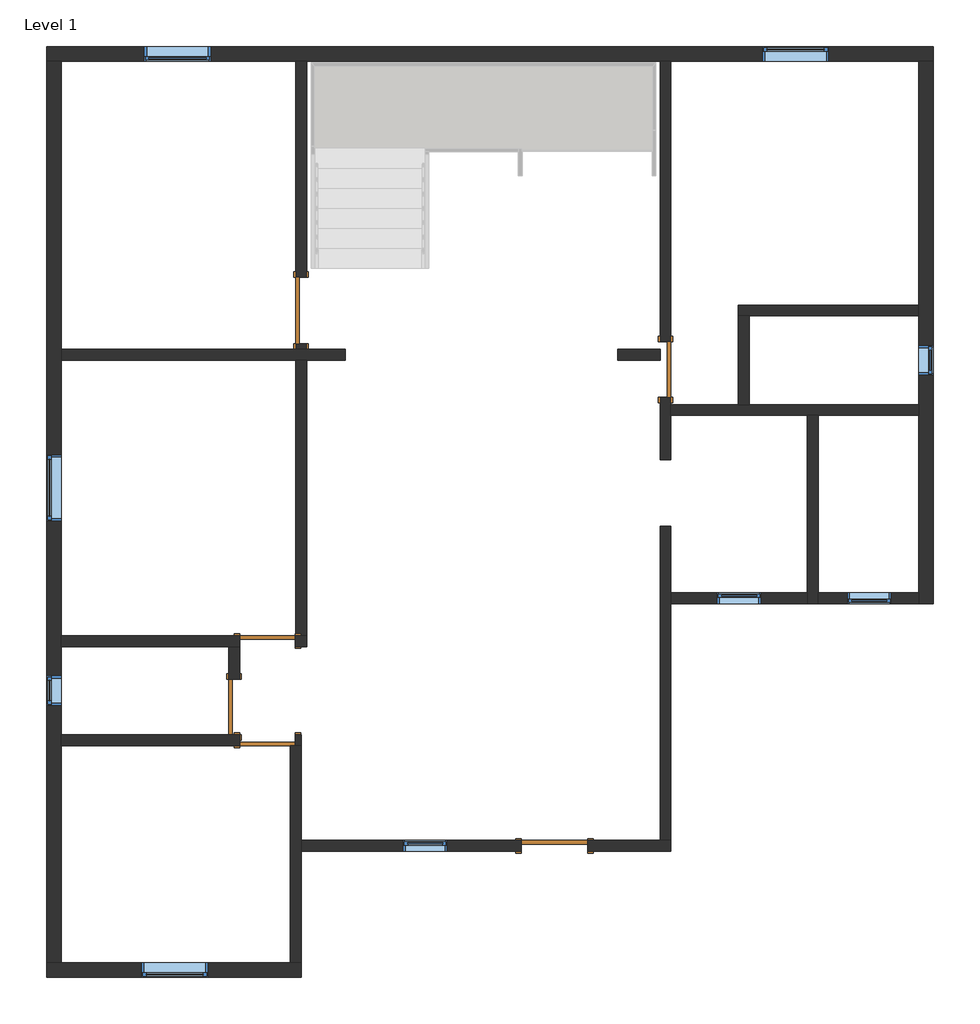
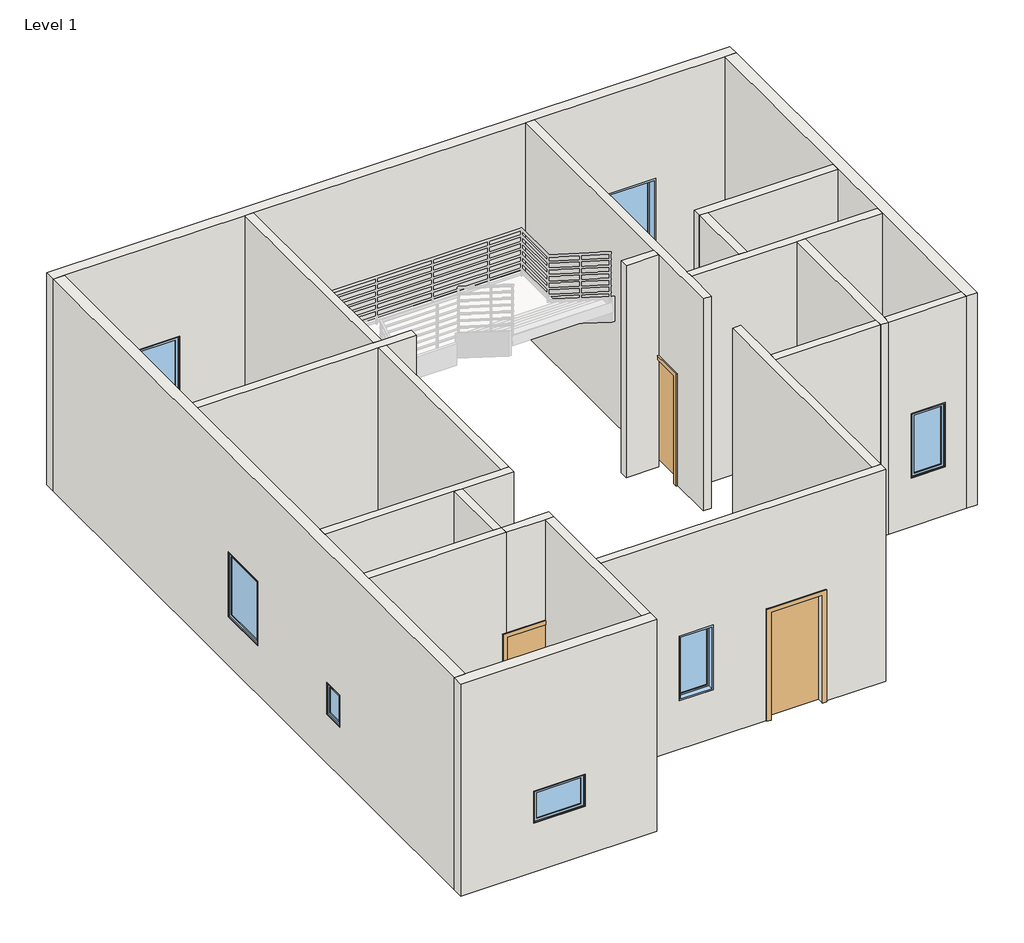
# One storey, part 1 of 3: 22 walls, 9 windows, 6 doors.
"""IFC4 building model written with IfcOpenShell, lengths in millimetres."""

from ifc_helpers import new_model, si_unit, frame, origin, origin_with_axes, place, context, project, spatial, polyline, outline, extrude, faceted_brep, transform, mapped, element, save
from components import m_single_flush_0762_x_2032mm_3f592dcc, m_single_flush_0762_x_2032mm_ffa3ef71, m_single_flush_0915_x_2032mm_d0c19338, m_single_flush_0915_x_2134mm_f3d7f739, m_fixed_0406_x_0610mm_8205b201, m_fixed_0610_x_1220mm_1758882d, m_fixed_0915_x_0610mm_70a843a6, m_fixed_0915_x_1220mm_488fb2fb

model = new_model("IFC4")

# Units and contexts
model_context = context("Model", 3, world=origin())
ifc_project = project(units=[si_unit("LENGTHUNIT", "METRE", prefix="MILLI")], contexts=[model_context])

# Site, building, storey
site = spatial("IfcSite", under=ifc_project)
building = spatial("IfcBuilding", under=site)
storey = spatial("IfcBuildingStorey", under=building, Name="Level 1", Elevation=0.0)

# Doors
placement = place(None, origin())
m_single_flush_0762_x_2032mm_shape = m_single_flush_0762_x_2032mm_3f592dcc(model_context)
element("IfcDoor", 1, ObjectType="M_Single-Flush : 0762 x 2032mm", at=placement, inside=storey, context=model_context, shape_type="MappedRepresentation", body=[
    mapped(m_single_flush_0762_x_2032mm_shape, transform((2439.4843899, 7347.685068, 0.0), x_axis=(0.0, -1.0, 0.0), y_axis=(1.0, 0.0, 0.0), z_axis=(0.0, 0.0, 1.0))),
])
element("IfcDoor", 2, ObjectType="M_Single-Flush : 0762 x 2032mm", at=placement, inside=storey, context=model_context, shape_type="MappedRepresentation", body=[
    mapped(m_single_flush_0762_x_2032mm_shape, transform((-3031.8906101, 3613.885068, 0.0), x_axis=(1.0, 0.0, 0.0), y_axis=(0.0, 1.0, 0.0), z_axis=(0.0, 0.0, 1.0))),
])
m_single_flush_0762_x_2032mm_2_shape = m_single_flush_0762_x_2032mm_ffa3ef71(model_context)
element("IfcDoor", 3, ObjectType="M_Single-Flush : 0762 x 2032mm", at=placement, inside=storey, context=model_context, shape_type="MappedRepresentation", body=[
    mapped(m_single_flush_0762_x_2032mm_2_shape, transform((-3492.2656101, 2707.035068, 0.0), x_axis=(0.0, -1.0, 0.0), y_axis=(1.0, 0.0, 0.0), z_axis=(0.0, 0.0, 1.0))),
])
element("IfcDoor", 4, ObjectType="M_Single-Flush : 0762 x 2032mm", at=placement, inside=storey, context=model_context, shape_type="MappedRepresentation", body=[
    mapped(m_single_flush_0762_x_2032mm_2_shape, transform((-3031.8906101, 2249.835068, 0.0), x_axis=(1.0, 0.0, 0.0), y_axis=(0.0, 1.0, 0.0), z_axis=(0.0, 0.0, 1.0))),
])
m_single_flush_0915_x_2032mm_shape = m_single_flush_0915_x_2032mm_d0c19338(model_context)
element("IfcDoor", 5, ObjectType="M_Single-Flush : 0915 x 2032mm", at=placement, inside=storey, context=model_context, shape_type="MappedRepresentation", body=[
    mapped(m_single_flush_0915_x_2032mm_shape, transform((915.4843899, 797.260068, 0.0), x_axis=(1.0, 0.0, 0.0), y_axis=(0.0, 1.0, 0.0), z_axis=(0.0, 0.0, 1.0))),
])
m_single_flush_0915_x_2134mm_shape = m_single_flush_0915_x_2134mm_f3d7f739(model_context)
element("IfcDoor", 6, ObjectType="M_Single-Flush : 0915 x 2134mm", at=placement, inside=storey, context=model_context, shape_type="MappedRepresentation", body=[
    mapped(m_single_flush_0915_x_2134mm_shape, transform((-2571.5156101, 8160.485068, 0.0), x_axis=(0.0, -1.0, 0.0), y_axis=(1.0, 0.0, 0.0), z_axis=(0.0, 0.0, 1.0))),
])

# Walls
element("IfcWall", 7, ObjectType="Generic - 150mm", at=placement, inside=storey, context=model_context, shape_type="Brep", body=[
    faceted_brep([(-5872.3156101, 7475.885068, 0.0), (-2646.5156101, 7475.885068, 0.0), (-2496.5156101, 7475.885068, 0.0), (-1963.1156101, 7475.885068, 0.0), (-1963.1156101, 7475.885068, 4000.0), (-2496.5156101, 7475.885068, 4000.0), (-2646.5156101, 7475.885068, 4000.0), (-5872.3156101, 7475.885068, 4000.0), (-5872.3156101, 7625.885068, 0.0), (-5872.3156101, 7625.885068, 4000.0), (-2646.5156101, 7625.885068, 4000.0), (-2496.5156101, 7625.885068, 4000.0), (-1963.1156101, 7625.885068, 4000.0), (-1963.1156101, 7625.885068, 0.0), (-2496.5156101, 7625.885068, 0.0), (-2646.5156101, 7625.885068, 0.0)], [[[0, 1, 2, 3, 4, 5, 6, 7]], [[8, 9, 10, 11, 12, 13, 14, 15]], [[3, 2, 1, 0, 8, 15, 14, 13]], [[4, 3, 13, 12]], [[7, 6, 5, 4, 12, 11, 10, 9]], [[0, 7, 9, 8]]]),
])
element("IfcWall", 8, ObjectType="Generic - 150mm", at=placement, inside=storey, context=model_context, shape_type="SweptSolid", body=[
    extrude(outline(polyline([(7702.985068, 2134.0), (7702.985068, 0.0), (7625.885068, 0.0), (7625.885068, 4000.0), (11589.885068, 4000.0), (11589.885068, 0.0), (8617.985068, 0.0), (8617.985068, 2134.0), (7702.985068, 2134.0)])), frame((-2646.5156101, 0.0, 0.0), z_axis=(1.0, 0.0, 0.0), x_axis=(0.0, 1.0, 0.0)), (0.0, 0.0, 1.0), 150.0),
])
element("IfcWall", 9, ObjectType="Generic - 150mm", at=placement, inside=storey, context=model_context, shape_type="Brep", body=[
    faceted_brep([(2364.4843899, 6966.685068, 2032.0), (2364.4843899, 6966.685068, 0.0), (2364.4843899, 6106.685068, 0.0), (2364.4843899, 6106.685068, 4000.0), (2364.4843899, 7475.885068, 4000.0), (2364.4843899, 7625.885068, 4000.0), (2364.4843899, 11589.885068, 4000.0), (2364.4843899, 11589.885068, 0.0), (2364.4843899, 7728.685068, 0.0), (2364.4843899, 7728.685068, 2032.0), (2514.4843899, 6106.685068, 0.0), (2514.4843899, 6716.285068, 0.0), (2514.4843899, 6866.285068, 0.0), (2514.4843899, 6966.685068, 0.0), (2514.4843899, 6966.685068, 2032.0), (2514.4843899, 7728.685068, 2032.0), (2514.4843899, 7728.685068, 0.0), (2514.4843899, 11589.885068, 0.0), (2514.4843899, 11589.885068, 4000.0), (2514.4843899, 6866.285068, 4000.0), (2514.4843899, 6716.285068, 4000.0), (2514.4843899, 6106.685068, 4000.0)], [[[0, 1, 2, 3, 4, 5, 6, 7, 8, 9]], [[10, 11, 12, 13, 14, 15, 16, 17, 18, 19, 20, 21]], [[8, 7, 17, 16]], [[2, 1, 13, 12, 11, 10]], [[3, 2, 10, 21]], [[6, 5, 4, 3, 21, 20, 19, 18]], [[7, 6, 18, 17]], [[14, 13, 1, 0]], [[15, 14, 0, 9]], [[16, 15, 9, 8]]]),
])
element("IfcWall", 10, ObjectType="Generic - 150mm", at=placement, inside=storey, context=model_context, shape_type="Brep", body=[
    faceted_brep([(3439.6343899, 8085.485068, 0.0), (3589.6343899, 8085.485068, 0.0), (5919.6843899, 8085.485068, 0.0), (5919.6843899, 8085.485068, 4000.0), (3589.6343899, 8085.485068, 4000.0), (3439.6343899, 8085.485068, 4000.0), (3439.6343899, 8235.485068, 0.0), (3439.6343899, 8235.485068, 4000.0), (5919.6843899, 8235.485068, 4000.0), (5919.6843899, 8235.485068, 0.0)], [[[0, 1, 2, 3, 4, 5]], [[6, 7, 8, 9]], [[2, 1, 0, 6, 9]], [[5, 4, 3, 8, 7]], [[3, 2, 9, 8]], [[0, 5, 7, 6]]]),
])
element("IfcWall", 11, ObjectType="Generic - 150mm", at=placement, inside=storey, context=model_context, shape_type="Brep", body=[
    faceted_brep([(-2496.5156101, 3688.885068, 0.0), (-2646.5156101, 3688.885068, 0.0), (-2650.8906101, 3688.885068, 0.0), (-2650.8906101, 3688.885068, 2032.0), (-3412.8906101, 3688.885068, 2032.0), (-3412.8906101, 3688.885068, 0.0), (-5872.3156101, 3688.885068, 0.0), (-5872.3156101, 3688.885068, 4000.0), (-2646.5156101, 3688.885068, 4000.0), (-2496.5156101, 3688.885068, 4000.0), (-2650.8906101, 3538.885068, 2032.0), (-2650.8906101, 3538.885068, 0.0), (-2496.5156101, 3538.885068, 0.0), (-2496.5156101, 3538.885068, 4000.0), (-3417.2656101, 3538.885068, 4000.0), (-3567.2656101, 3538.885068, 4000.0), (-5872.3156101, 3538.885068, 4000.0), (-5872.3156101, 3538.885068, 0.0), (-3567.2656101, 3538.885068, 0.0), (-3417.2656101, 3538.885068, 0.0), (-3412.8906101, 3538.885068, 0.0), (-3412.8906101, 3538.885068, 2032.0)], [[[0, 1, 2, 3, 4, 5, 6, 7, 8, 9]], [[10, 11, 12, 13, 14, 15, 16, 17, 18, 19, 20, 21]], [[12, 11, 2, 1, 0]], [[20, 19, 18, 17, 6, 5]], [[9, 8, 7, 16, 15, 14, 13]], [[7, 6, 17, 16]], [[0, 9, 13, 12]], [[3, 2, 11, 10]], [[4, 3, 10, 21]], [[5, 4, 21, 20]]]),
])
element("IfcWall", 12, ObjectType="Generic - 150mm", at=placement, inside=storey, context=model_context, shape_type="SweptSolid", body=[
    extrude(outline(polyline([(3439.6343899, 6866.285068), (3439.6343899, 8085.485068), (3589.6343899, 8085.485068), (3589.6343899, 6866.285068), (3439.6343899, 6866.285068)])), origin_with_axes(), (0.0, 0.0, 1.0), 4000.0),
])
element("IfcWall", 13, ObjectType="Generic - 150mm", at=placement, inside=storey, context=model_context, shape_type="Brep", body=[
    faceted_brep([(2514.4843899, 6716.285068, 0.0), (4390.1343899, 6716.285068, 0.0), (4540.1343899, 6716.285068, 0.0), (5919.6843899, 6716.285068, 0.0), (5919.6843899, 6716.285068, 4000.0), (4540.1343899, 6716.285068, 4000.0), (4390.1343899, 6716.285068, 4000.0), (2514.4843899, 6716.285068, 4000.0), (2514.4843899, 6866.285068, 0.0), (2514.4843899, 6866.285068, 4000.0), (3439.6343899, 6866.285068, 4000.0), (3589.6343899, 6866.285068, 4000.0), (5919.6843899, 6866.285068, 4000.0), (5919.6843899, 6866.285068, 0.0), (3589.6343899, 6866.285068, 0.0), (3439.6343899, 6866.285068, 0.0)], [[[0, 1, 2, 3, 4, 5, 6, 7]], [[8, 9, 10, 11, 12, 13, 14, 15]], [[3, 2, 1, 0, 8, 15, 14, 13]], [[7, 6, 5, 4, 12, 11, 10, 9]], [[4, 3, 13, 12]], [[0, 7, 9, 8]]]),
])
element("IfcWall", 14, ObjectType="Generic - 150mm", at=placement, inside=storey, context=model_context, shape_type="Brep", body=[
    faceted_brep([(4390.1343899, 6716.285068, 0.0), (4390.1343899, 4277.885068, 0.0), (4390.1343899, 4127.885068, 0.0), (4390.1343899, 4127.885068, 4000.0), (4390.1343899, 4277.885068, 4000.0), (4390.1343899, 6716.285068, 4000.0), (4540.1343899, 6716.285068, 0.0), (4540.1343899, 6716.285068, 4000.0), (4540.1343899, 4277.885068, 4000.0), (4540.1343899, 4127.885068, 4000.0), (4540.1343899, 4127.885068, 0.0), (4540.1343899, 4277.885068, 0.0)], [[[0, 1, 2, 3, 4, 5]], [[6, 7, 8, 9, 10, 11]], [[2, 1, 0, 6, 11, 10]], [[5, 4, 3, 9, 8, 7]], [[0, 5, 7, 6]], [[3, 2, 10, 9]]]),
])
element("IfcWall", 15, ObjectType="Generic - 150mm", at=placement, inside=storey, context=model_context, shape_type="SweptSolid", body=[
    extrude(outline(polyline([(0.0, 4540.1343899), (0.0, 5919.6843899), (4000.0, 5919.6843899), (4000.0, 4540.1343899), (0.0, 4540.1343899)]), holes=[polyline([(915.0, 5547.4093899), (915.0, 4937.4093899), (2135.0, 4937.4093899), (2135.0, 5547.4093899), (915.0, 5547.4093899)])]), frame((0.0, 4127.885068, 0.0), z_axis=(0.0, 1.0, 0.0), x_axis=(0.0, 0.0, 1.0)), (0.0, 0.0, 1.0), 150.0),
])
element("IfcWall", 16, ObjectType="Generic - 150mm", at=placement, inside=storey, context=model_context, shape_type="SweptSolid", body=[
    extrude(outline(polyline([(0.0, 4390.1343899), (4000.0, 4390.1343899), (4000.0, 2514.4843899), (0.0, 2514.4843899), (0.0, 4390.1343899)]), holes=[polyline([(915.0, 3147.3093899), (2135.0, 3147.3093899), (2135.0, 3757.3093899), (915.0, 3757.3093899), (915.0, 3147.3093899)])]), frame((0.0, 4127.885068, 0.0), z_axis=(0.0, 1.0, 0.0), x_axis=(0.0, 0.0, 1.0)), (0.0, 0.0, 1.0), 150.0),
])
element("IfcWall", 17, ObjectType="Generic - 150mm", at=placement, inside=storey, context=model_context, shape_type="Brep", body=[
    faceted_brep([(2514.4843899, 872.260068, 0.0), (2514.4843899, 4127.885068, 0.0), (2514.4843899, 4277.885068, 0.0), (2514.4843899, 5194.685068, 0.0), (2514.4843899, 5194.685068, 4000.0), (2514.4843899, 4277.885068, 4000.0), (2514.4843899, 4127.885068, 4000.0), (2514.4843899, 872.260068, 4000.0), (2364.4843899, 872.260068, 0.0), (2364.4843899, 872.260068, 4000.0), (2364.4843899, 5194.685068, 4000.0), (2364.4843899, 5194.685068, 0.0)], [[[0, 1, 2, 3, 4, 5, 6, 7]], [[8, 9, 10, 11]], [[3, 2, 1, 0, 8, 11]], [[4, 3, 11, 10]], [[7, 6, 5, 4, 10, 9]], [[0, 7, 9, 8]]]),
])
element("IfcWall", 18, ObjectType="Generic - 150mm", at=placement, inside=storey, context=model_context, shape_type="Brep", body=[
    faceted_brep([(-5872.3156101, 2174.835068, 0.0), (-3417.2656101, 2174.835068, 0.0), (-3417.2656101, 2174.835068, 4000.0), (-5872.3156101, 2174.835068, 4000.0), (-5872.3156101, 2324.835068, 0.0), (-5872.3156101, 2324.835068, 4000.0), (-3567.2656101, 2324.835068, 4000.0), (-3417.2656101, 2324.835068, 4000.0), (-3417.2656101, 2324.835068, 0.0), (-3567.2656101, 2324.835068, 0.0)], [[[0, 1, 2, 3]], [[4, 5, 6, 7, 8, 9]], [[1, 0, 4, 9, 8]], [[3, 2, 7, 6, 5]], [[0, 3, 5, 4]], [[2, 1, 8, 7]]]),
])
element("IfcWall", 19, ObjectType="Generic - 150mm", at=placement, inside=storey, context=model_context, shape_type="SweptSolid", body=[
    extrude(outline(polyline([(2326.035068, 2032.0), (2326.035068, 0.0), (2324.835068, 0.0), (2324.835068, 4000.0), (3538.885068, 4000.0), (3538.885068, 0.0), (3088.035068, 0.0), (3088.035068, 2032.0), (2326.035068, 2032.0)])), frame((-3567.2656101, 0.0, 0.0), z_axis=(1.0, 0.0, 0.0), x_axis=(0.0, 1.0, 0.0)), (0.0, 0.0, 1.0), 150.0),
])
element("IfcWall", 20, ObjectType="Generic - 150mm", at=placement, inside=storey, context=model_context, shape_type="Brep", body=[
    faceted_brep([(-2571.5156101, 2324.835068, 0.0), (-2650.8906101, 2324.835068, 0.0), (-2650.8906101, 2324.835068, 2032.0), (-3412.8906101, 2324.835068, 2032.0), (-3412.8906101, 2324.835068, 0.0), (-3417.2656101, 2324.835068, 0.0), (-3417.2656101, 2324.835068, 4000.0), (-2571.5156101, 2324.835068, 4000.0), (-2650.8906101, 2174.835068, 2032.0), (-2650.8906101, 2174.835068, 0.0), (-2571.5156101, 2174.835068, 0.0), (-2571.5156101, 2174.835068, 4000.0), (-2721.5156101, 2174.835068, 4000.0), (-3417.2656101, 2174.835068, 4000.0), (-3417.2656101, 2174.835068, 0.0), (-3412.8906101, 2174.835068, 0.0), (-3412.8906101, 2174.835068, 2032.0)], [[[0, 1, 2, 3, 4, 5, 6, 7]], [[8, 9, 10, 11, 12, 13, 14, 15, 16]], [[15, 14, 5, 4]], [[10, 9, 1, 0]], [[7, 6, 13, 12, 11]], [[6, 5, 14, 13]], [[0, 7, 11, 10]], [[2, 1, 9, 8]], [[3, 2, 8, 16]], [[4, 3, 16, 15]]]),
])
element("IfcWall", 21, ObjectType="Generic - 150mm", at=placement, inside=storey, context=model_context, shape_type="SweptSolid", body=[
    extrude(outline(polyline([(-2646.5156101, 3688.885068), (-2646.5156101, 7475.885068), (-2496.5156101, 7475.885068), (-2496.5156101, 3688.885068), (-2646.5156101, 3688.885068)])), origin_with_axes(), (0.0, 0.0, 1.0), 4000.0),
])
element("IfcWall", 22, ObjectType="Generic - 150mm", at=placement, inside=storey, context=model_context, shape_type="Brep", body=[
    faceted_brep([(-2721.5156101, 2174.835068, 0.0), (-2721.5156101, -811.714932, 0.0), (-2721.5156101, -811.714932, 4000.0), (-2721.5156101, 2174.835068, 4000.0), (-2571.5156101, 2174.835068, 0.0), (-2571.5156101, 2174.835068, 4000.0), (-2571.5156101, 872.260068, 4000.0), (-2571.5156101, 722.260068, 4000.0), (-2571.5156101, -811.714932, 4000.0), (-2571.5156101, -811.714932, 0.0), (-2571.5156101, 722.260068, 0.0), (-2571.5156101, 872.260068, 0.0)], [[[0, 1, 2, 3]], [[4, 5, 6, 7, 8, 9, 10, 11]], [[1, 0, 4, 11, 10, 9]], [[3, 2, 8, 7, 6, 5]], [[0, 3, 5, 4]], [[2, 1, 9, 8]]]),
])
element("IfcWall", 23, ObjectType="Generic - 150mm", at=placement, inside=storey, context=model_context, shape_type="Brep", body=[
    faceted_brep([(1372.9843899, 722.260068, 2032.0), (1372.9843899, 722.260068, 0.0), (2514.4843899, 722.260068, 0.0), (2514.4843899, 722.260068, 4000.0), (-2571.5156101, 722.260068, 4000.0), (-2571.5156101, 722.260068, 0.0), (457.9843899, 722.260068, 0.0), (457.9843899, 722.260068, 2032.0), (-1170.5156101, 722.260068, 915.0), (-1170.5156101, 722.260068, 2135.0), (-560.5156101, 722.260068, 2135.0), (-560.5156101, 722.260068, 915.0), (2514.4843899, 872.260068, 0.0), (2364.4843899, 872.260068, 0.0), (1372.9843899, 872.260068, 0.0), (1372.9843899, 872.260068, 2032.0), (457.9843899, 872.260068, 2032.0), (457.9843899, 872.260068, 0.0), (-2571.5156101, 872.260068, 0.0), (-2571.5156101, 872.260068, 4000.0), (2364.4843899, 872.260068, 4000.0), (2514.4843899, 872.260068, 4000.0), (-1170.5156101, 872.260068, 915.0), (-560.5156101, 872.260068, 915.0), (-560.5156101, 872.260068, 2135.0), (-1170.5156101, 872.260068, 2135.0)], [[[0, 1, 2, 3, 4, 5, 6, 7], [8, 9, 10, 11]], [[12, 13, 14, 15, 16, 17, 18, 19, 20, 21], [22, 23, 24, 25]], [[6, 5, 18, 17]], [[2, 1, 14, 13, 12]], [[4, 3, 21, 20, 19]], [[5, 4, 19, 18]], [[3, 2, 12, 21]], [[15, 14, 1, 0]], [[16, 15, 0, 7]], [[17, 16, 7, 6]], [[9, 8, 22, 25]], [[10, 9, 25, 24]], [[11, 10, 24, 23]], [[8, 11, 23, 22]]]),
])
element("IfcWall", 24, ObjectType="Generic - 150mm", at=placement, inside=storey, context=model_context, shape_type="SweptSolid", body=[
    extrude(outline(polyline([(1780.2843899, 7625.885068), (2364.4843899, 7625.885068), (2364.4843899, 7475.885068), (1780.2843899, 7475.885068), (1780.2843899, 7625.885068)])), origin_with_axes(), (0.0, 0.0, 1.0), 4000.0),
])
element("IfcWall", 25, ObjectType="Generic - 200mm", at=placement, inside=storey, context=model_context, shape_type="Brep", body=[
    faceted_brep([(-6072.3156101, 11589.885068, 0.0), (-5872.3156101, 11589.885068, 0.0), (-2646.5156101, 11589.885068, 0.0), (-2496.5156101, 11589.885068, 0.0), (2364.4843899, 11589.885068, 0.0), (2514.4843899, 11589.885068, 0.0), (5919.6843899, 11589.885068, 0.0), (6119.6843899, 11589.885068, 0.0), (6119.6843899, 11589.885068, 4000.0), (5919.6843899, 11589.885068, 4000.0), (2514.4843899, 11589.885068, 4000.0), (2364.4843899, 11589.885068, 4000.0), (-2496.5156101, 11589.885068, 4000.0), (-2646.5156101, 11589.885068, 4000.0), (-5872.3156101, 11589.885068, 4000.0), (-6072.3156101, 11589.885068, 4000.0), (-3814.4156101, 11589.885068, 915.0), (-4729.4156101, 11589.885068, 915.0), (-4729.4156101, 11589.885068, 2135.0), (-3814.4156101, 11589.885068, 2135.0), (3772.0843899, 11589.885068, 915.0), (3772.0843899, 11589.885068, 2135.0), (4687.0843899, 11589.885068, 2135.0), (4687.0843899, 11589.885068, 915.0), (-6072.3156101, 11789.885068, 0.0), (-6072.3156101, 11789.885068, 4000.0), (6119.6843899, 11789.885068, 4000.0), (6119.6843899, 11789.885068, 0.0), (-3814.4156101, 11789.885068, 915.0), (-3814.4156101, 11789.885068, 2135.0), (-4729.4156101, 11789.885068, 2135.0), (-4729.4156101, 11789.885068, 915.0), (3772.0843899, 11789.885068, 915.0), (4687.0843899, 11789.885068, 915.0), (4687.0843899, 11789.885068, 2135.0), (3772.0843899, 11789.885068, 2135.0)], [[[0, 1, 2, 3, 4, 5, 6, 7, 8, 9, 10, 11, 12, 13, 14, 15], [16, 17, 18, 19], [20, 21, 22, 23]], [[24, 25, 26, 27], [28, 29, 30, 31], [32, 33, 34, 35]], [[7, 6, 5, 4, 3, 2, 1, 0, 24, 27]], [[15, 14, 13, 12, 11, 10, 9, 8, 26, 25]], [[8, 7, 27, 26]], [[0, 15, 25, 24]], [[29, 28, 16, 19]], [[30, 29, 19, 18]], [[31, 30, 18, 17]], [[28, 31, 17, 16]], [[21, 20, 32, 35]], [[22, 21, 35, 34]], [[23, 22, 34, 33]], [[20, 23, 33, 32]]]),
])
element("IfcWall", 26, ObjectType="Generic - 200mm", at=placement, inside=storey, context=model_context, shape_type="Brep", body=[
    faceted_brep([(5919.6843899, 11589.885068, 0.0), (5919.6843899, 8235.485068, 0.0), (5919.6843899, 8085.485068, 0.0), (5919.6843899, 6866.285068, 0.0), (5919.6843899, 6716.285068, 0.0), (5919.6843899, 4277.885068, 0.0), (5919.6843899, 4127.885068, 0.0), (5919.6843899, 4127.885068, 4000.0), (5919.6843899, 4277.885068, 4000.0), (5919.6843899, 6716.285068, 4000.0), (5919.6843899, 6866.285068, 4000.0), (5919.6843899, 8085.485068, 4000.0), (5919.6843899, 8235.485068, 4000.0), (5919.6843899, 11589.885068, 4000.0), (5919.6843899, 7678.885068, 915.0), (5919.6843899, 7678.885068, 1525.0), (5919.6843899, 7272.885068, 1525.0), (5919.6843899, 7272.885068, 915.0), (6119.6843899, 11589.885068, 0.0), (6119.6843899, 11589.885068, 4000.0), (6119.6843899, 4127.885068, 4000.0), (6119.6843899, 4127.885068, 0.0), (6119.6843899, 7678.885068, 915.0), (6119.6843899, 7272.885068, 915.0), (6119.6843899, 7272.885068, 1525.0), (6119.6843899, 7678.885068, 1525.0)], [[[0, 1, 2, 3, 4, 5, 6, 7, 8, 9, 10, 11, 12, 13], [14, 15, 16, 17]], [[18, 19, 20, 21], [22, 23, 24, 25]], [[6, 5, 4, 3, 2, 1, 0, 18, 21]], [[13, 12, 11, 10, 9, 8, 7, 20, 19]], [[0, 13, 19, 18]], [[7, 6, 21, 20]], [[15, 14, 22, 25]], [[16, 15, 25, 24]], [[17, 16, 24, 23]], [[14, 17, 23, 22]]]),
])
element("IfcWall", 27, ObjectType="Generic - 200mm", at=placement, inside=storey, context=model_context, shape_type="Brep", body=[
    faceted_brep([(-2571.5156101, -811.714932, 0.0), (-2721.5156101, -811.714932, 0.0), (-5872.3156101, -811.714932, 0.0), (-6072.3156101, -811.714932, 0.0), (-6072.3156101, -811.714932, 4000.0), (-5872.3156101, -811.714932, 4000.0), (-2721.5156101, -811.714932, 4000.0), (-2571.5156101, -811.714932, 4000.0), (-3851.9156101, -811.714932, 915.0), (-3851.9156101, -811.714932, 1525.0), (-4766.9156101, -811.714932, 1525.0), (-4766.9156101, -811.714932, 915.0), (-2571.5156101, -1011.714932, 0.0), (-2571.5156101, -1011.714932, 4000.0), (-6072.3156101, -1011.714932, 4000.0), (-6072.3156101, -1011.714932, 0.0), (-3851.9156101, -1011.714932, 915.0), (-4766.9156101, -1011.714932, 915.0), (-4766.9156101, -1011.714932, 1525.0), (-3851.9156101, -1011.714932, 1525.0)], [[[0, 1, 2, 3, 4, 5, 6, 7], [8, 9, 10, 11]], [[12, 13, 14, 15], [16, 17, 18, 19]], [[3, 2, 1, 0, 12, 15]], [[7, 6, 5, 4, 14, 13]], [[4, 3, 15, 14]], [[0, 7, 13, 12]], [[9, 8, 16, 19]], [[10, 9, 19, 18]], [[11, 10, 18, 17]], [[8, 11, 17, 16]]]),
])
element("IfcWall", 28, ObjectType="Generic - 200mm", at=placement, inside=storey, context=model_context, shape_type="Brep", body=[
    faceted_brep([(-5872.3156101, -811.714932, 0.0), (-5872.3156101, 2174.835068, 0.0), (-5872.3156101, 2324.835068, 0.0), (-5872.3156101, 3538.885068, 0.0), (-5872.3156101, 3688.885068, 0.0), (-5872.3156101, 7475.885068, 0.0), (-5872.3156101, 7625.885068, 0.0), (-5872.3156101, 11589.885068, 0.0), (-5872.3156101, 11589.885068, 4000.0), (-5872.3156101, 7625.885068, 4000.0), (-5872.3156101, 7475.885068, 4000.0), (-5872.3156101, 3688.885068, 4000.0), (-5872.3156101, 3538.885068, 4000.0), (-5872.3156101, 2324.835068, 4000.0), (-5872.3156101, 2174.835068, 4000.0), (-5872.3156101, -811.714932, 4000.0), (-5872.3156101, 2728.860068, 915.0), (-5872.3156101, 2728.860068, 1525.0), (-5872.3156101, 3134.860068, 1525.0), (-5872.3156101, 3134.860068, 915.0), (-5872.3156101, 5264.585068, 915.0), (-5872.3156101, 5264.585068, 2135.0), (-5872.3156101, 6179.585068, 2135.0), (-5872.3156101, 6179.585068, 915.0), (-6072.3156101, -811.714932, 0.0), (-6072.3156101, -811.714932, 4000.0), (-6072.3156101, 11589.885068, 4000.0), (-6072.3156101, 11589.885068, 0.0), (-6072.3156101, 2728.860068, 915.0), (-6072.3156101, 3134.860068, 915.0), (-6072.3156101, 3134.860068, 1525.0), (-6072.3156101, 2728.860068, 1525.0), (-6072.3156101, 5264.585068, 915.0), (-6072.3156101, 6179.585068, 915.0), (-6072.3156101, 6179.585068, 2135.0), (-6072.3156101, 5264.585068, 2135.0)], [[[0, 1, 2, 3, 4, 5, 6, 7, 8, 9, 10, 11, 12, 13, 14, 15], [16, 17, 18, 19], [20, 21, 22, 23]], [[24, 25, 26, 27], [28, 29, 30, 31], [32, 33, 34, 35]], [[7, 6, 5, 4, 3, 2, 1, 0, 24, 27]], [[15, 14, 13, 12, 11, 10, 9, 8, 26, 25]], [[0, 15, 25, 24]], [[8, 7, 27, 26]], [[17, 16, 28, 31]], [[18, 17, 31, 30]], [[19, 18, 30, 29]], [[16, 19, 29, 28]], [[21, 20, 32, 35]], [[22, 21, 35, 34]], [[23, 22, 34, 33]], [[20, 23, 33, 32]]]),
])

# Windows
m_fixed_0406_x_0610mm_shape = m_fixed_0406_x_0610mm_8205b201(model_context)
element("IfcWindow", 29, ObjectType="M_Fixed : 0406 x 0610mm", at=placement, inside=storey, context=model_context, shape_type="MappedRepresentation", body=[
    mapped(m_fixed_0406_x_0610mm_shape, transform((-5959.3156101, 2931.860068, 0.0), x_axis=(0.0, 1.0, 0.0), y_axis=(-1.0, 0.0, 0.0), z_axis=(0.0, 0.0, 1.0))),
])
element("IfcWindow", 30, ObjectType="M_Fixed : 0406 x 0610mm", at=placement, inside=storey, context=model_context, shape_type="MappedRepresentation", body=[
    mapped(m_fixed_0406_x_0610mm_shape, transform((6006.6843899, 7475.885068, 0.0), x_axis=(0.0, -1.0, 0.0), y_axis=(1.0, 0.0, 0.0), z_axis=(0.0, 0.0, 1.0))),
])
m_fixed_0610_x_1220mm_shape = m_fixed_0610_x_1220mm_1758882d(model_context)
element("IfcWindow", 31, ObjectType="M_Fixed : 0610 x 1220mm", at=placement, inside=storey, context=model_context, shape_type="MappedRepresentation", body=[
    mapped(m_fixed_0610_x_1220mm_shape, transform((3452.3093899, 4189.885068, 0.0), x_axis=(1.0, 0.0, 0.0), y_axis=(0.0, 1.0, 0.0), z_axis=(0.0, 0.0, 1.0))),
])
element("IfcWindow", 32, ObjectType="M_Fixed : 0610 x 1220mm", at=placement, inside=storey, context=model_context, shape_type="MappedRepresentation", body=[
    mapped(m_fixed_0610_x_1220mm_shape, transform((5242.4093899, 4215.885068, 0.0), x_axis=(-1.0, 0.0, 0.0), y_axis=(0.0, -1.0, 0.0), z_axis=(0.0, 0.0, 1.0))),
])
element("IfcWindow", 33, ObjectType="M_Fixed : 0610 x 1220mm", at=placement, inside=storey, context=model_context, shape_type="MappedRepresentation", body=[
    mapped(m_fixed_0610_x_1220mm_shape, transform((-865.5156101, 784.260068, 0.0), x_axis=(1.0, 0.0, 0.0), y_axis=(0.0, 1.0, 0.0), z_axis=(0.0, 0.0, 1.0))),
])
m_fixed_0915_x_0610mm_shape = m_fixed_0915_x_0610mm_70a843a6(model_context)
element("IfcWindow", 34, ObjectType="M_Fixed : 0915 x 0610mm", at=placement, inside=storey, context=model_context, shape_type="MappedRepresentation", body=[
    mapped(m_fixed_0915_x_0610mm_shape, transform((-4309.4156101, -898.714932, 0.0), x_axis=(-1.0, 0.0, 0.0), y_axis=(0.0, -1.0, 0.0), z_axis=(0.0, 0.0, 1.0))),
])
m_fixed_0915_x_1220mm_shape = m_fixed_0915_x_1220mm_488fb2fb(model_context)
element("IfcWindow", 35, ObjectType="M_Fixed : 0915 x 1220mm", at=placement, inside=storey, context=model_context, shape_type="MappedRepresentation", body=[
    mapped(m_fixed_0915_x_1220mm_shape, transform((-5959.3156101, 5722.085068, 0.0), x_axis=(0.0, 1.0, 0.0), y_axis=(-1.0, 0.0, 0.0), z_axis=(0.0, 0.0, 1.0))),
])
element("IfcWindow", 36, ObjectType="M_Fixed : 0915 x 1220mm", at=placement, inside=storey, context=model_context, shape_type="MappedRepresentation", body=[
    mapped(m_fixed_0915_x_1220mm_shape, transform((-4271.9156101, 11702.885068, 0.0), x_axis=(-1.0, 0.0, 0.0), y_axis=(0.0, -1.0, 0.0), z_axis=(0.0, 0.0, 1.0))),
])
element("IfcWindow", 37, ObjectType="M_Fixed : 0915 x 1220mm", at=placement, inside=storey, context=model_context, shape_type="MappedRepresentation", body=[
    mapped(m_fixed_0915_x_1220mm_shape, transform((4229.5843899, 11676.885068, 0.0), x_axis=(1.0, 0.0, 0.0), y_axis=(0.0, 1.0, 0.0), z_axis=(0.0, 0.0, 1.0))),
])

save(model, "model.ifc")

# Revit data of these elements
# Type "M_Single-Flush : 0762 x 2032mm"
#   Type Mark = "19"
#   Thickness = 51 mm
#   Height = 2032 mm
#   Trim Projection Ext = 25 mm
#   Trim Projection Int = 25 mm
#   Trim Width = 76 mm
#   Width = 762 mm
#   Door Material = Door - Panel
#   Frame Material = Door - Frame
#   Function = (empty or 0)
#   Wall Closure = (empty or 0)
# Type "M_Single-Flush : 0915 x 2032mm"
#   Type Mark = "20"
#   Thickness = 51 mm
#   Height = 2032 mm
#   Trim Projection Ext = 25 mm
#   Trim Projection Int = 25 mm
#   Trim Width = 76 mm
#   Width = 915 mm
#   Door Material = Door - Panel
#   Frame Material = Door - Frame
#   Function = (empty or 0)
#   Wall Closure = (empty or 0)
# Type "M_Single-Flush : 0915 x 2134mm"
#   Type Mark = "15"
#   Thickness = 51 mm
#   Height = 2134 mm
#   Trim Projection Ext = 25 mm
#   Trim Projection Int = 25 mm
#   Trim Width = 76 mm
#   Width = 915 mm
#   Door Material = Door - Panel
#   Frame Material = Door - Frame
#   Function = (empty or 0)
#   Wall Closure = (empty or 0)
# Type "Generic - 150mm"
#   Layers, outside or top first: 150 mm no material (function 1)
# Type "Generic - 200mm"
#   Layers, outside or top first: 200 mm no material (function 1)
# Type "M_Fixed : 0406 x 0610mm"
#   Type Mark = "10"
#   Height = 610 mm
#   Default Sill Height = 915 mm
#   Width = 406 mm
#   Window Inset = 19 mm
#   Frame Exterior Material = Sash
#   Frame Interior Material = Sash
#   Glass Pane Material = Glass
#   Sash = Sash
#   Wall Closure = (empty or 0)
# Type "M_Fixed : 0610 x 1220mm"
#   Type Mark = "13"
#   Height = 1220 mm
#   Default Sill Height = 915 mm
#   Width = 610 mm
#   Window Inset = 19 mm
#   Frame Exterior Material = Sash
#   Frame Interior Material = Sash
#   Glass Pane Material = Glass
#   Sash = Sash
#   Wall Closure = (empty or 0)
# Type "M_Fixed : 0915 x 0610mm"
#   Type Mark = "14"
#   Height = 610 mm
#   Default Sill Height = 915 mm
#   Width = 915 mm
#   Window Inset = 19 mm
#   Frame Exterior Material = Sash
#   Frame Interior Material = Sash
#   Glass Pane Material = Glass
#   Sash = Sash
#   Wall Closure = (empty or 0)
# Type "M_Fixed : 0915 x 1220mm"
#   Type Mark = "15"
#   Height = 1220 mm
#   Default Sill Height = 915 mm
#   Width = 915 mm
#   Window Inset = 19 mm
#   Frame Exterior Material = Sash
#   Frame Interior Material = Sash
#   Glass Pane Material = Glass
#   Sash = Sash
#   Wall Closure = (empty or 0)
# Elements 1, 2, 3, 4 (IfcDoor, "M_Single-Flush : 0762 x 2032mm")
#   Phase Created = New Construction
#   Materials on its faces: "Door - Frame", "Door - Panel"
# Element 5 (IfcDoor, "M_Single-Flush : 0915 x 2032mm")
#   Phase Created = New Construction
#   Materials on its faces: "Door - Frame", "Door - Panel"
# Element 6 (IfcDoor, "M_Single-Flush : 0915 x 2134mm")
#   Phase Created = New Construction
#   Materials on its faces: "Door - Frame", "Door - Panel"
# Elements 7, 8, 9, 10, 11, 12, 13, 14, 15, 16, 17, 18, 19, 20, 21, 22, 23, 24 (IfcWall, "Generic - 150mm")
#   Top Offset = 0 mm
#   Base Offset = 0 mm
#   wall height = 4000 mm
#   Phase Created = New Construction
#   Base Constraint = Level 1
#   Top Constraint = Level 2
#   Materials on its faces: "Default Wall"
# Elements 25, 26, 27, 28 (IfcWall, "Generic - 200mm")
#   Top Offset = 0 mm
#   Base Offset = 0 mm
#   wall height = 4000 mm
#   Phase Created = New Construction
#   Base Constraint = Level 1
#   Top Constraint = Level 2
#   Materials on its faces: "Default Wall"
# Element 29 (IfcWindow, "M_Fixed : 0406 x 0610mm")
#   Mark = "6"
#   Phase Created = New Construction
#   Materials on its faces: "Sash", "Glass"
# Element 30 (IfcWindow, "M_Fixed : 0406 x 0610mm")
#   Mark = "7"
#   Phase Created = New Construction
#   Materials on its faces: "Sash", "Glass"
# Element 31 (IfcWindow, "M_Fixed : 0610 x 1220mm")
#   Mark = "11"
#   Phase Created = New Construction
#   Materials on its faces: "Sash", "Glass"
# Element 32 (IfcWindow, "M_Fixed : 0610 x 1220mm")
#   Mark = "12"
#   Phase Created = New Construction
#   Materials on its faces: "Sash", "Glass"
# Element 33 (IfcWindow, "M_Fixed : 0610 x 1220mm")
#   Mark = "13"
#   Phase Created = New Construction
#   Materials on its faces: "Sash", "Glass"
# Element 34 (IfcWindow, "M_Fixed : 0915 x 0610mm")
#   Mark = "14"
#   Phase Created = New Construction
#   Materials on its faces: "Sash", "Glass"
# Element 35 (IfcWindow, "M_Fixed : 0915 x 1220mm")
#   Mark = "8"
#   Phase Created = New Construction
#   Materials on its faces: "Sash", "Glass"
# Element 36 (IfcWindow, "M_Fixed : 0915 x 1220mm")
#   Mark = "9"
#   Phase Created = New Construction
#   Materials on its faces: "Sash", "Glass"
# Element 37 (IfcWindow, "M_Fixed : 0915 x 1220mm")
#   Mark = "10"
#   Phase Created = New Construction
#   Materials on its faces: "Sash", "Glass"
# Materials
#   "Door - Panel": class "Wood", colour RGB 114 82 51, transparency 0
#   "Door - Frame": colour RGB 153 76 43, transparency 0
#   "Sash": class "Wood", colour RGB 136 99 55, transparency 0
#   "Glass": class "Glass", colour RGB 218 227 224, transparency 0.85, Description = "Soda Lime Glass", Cost = 0
#   "Default Wall": colour RGB 80 80 80, transparency 0
